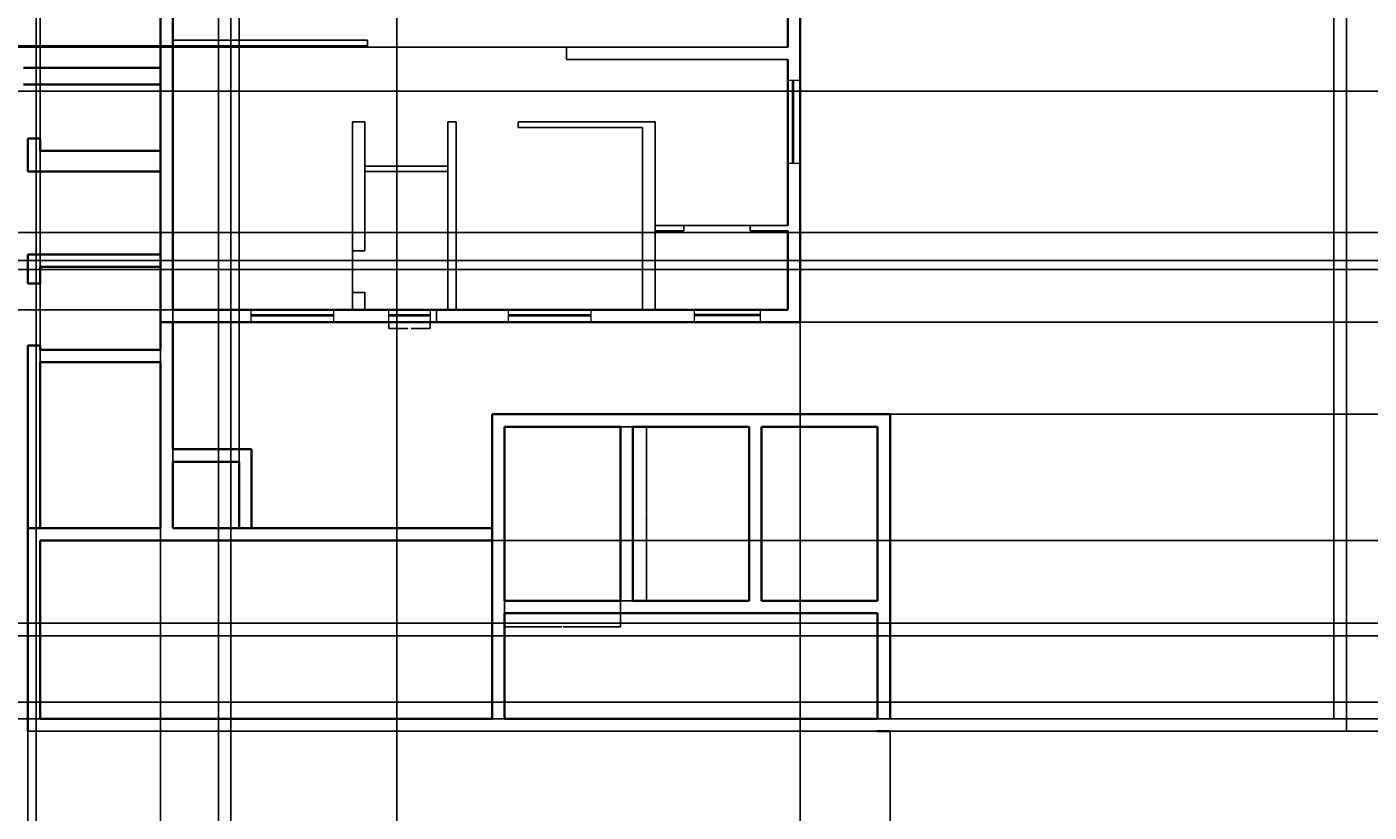
# Model space of a CAD drawing. Units: inches. Extents: x 2029 to 8798, y 1998 to 6373.
# Tile 5 of 11: x 2855 to 3826, y 4599 to 5168. Entities that reach past the tile are written whole.
import ezdxf

# ---------------------------------------------------------------- set-up
doc = ezdxf.new("R2010")
doc.units = ezdxf.units.IN
for name, color, linetype, lineweight in [('A-ANNO-DIMS', 2, 'Continuous', 18), ('A-GLAZ', 4, 'Continuous', 18), ('A-WALL-CIRC', 7, 'Continuous', 25), ('A-WALL-CORE', 7, 'Continuous', 35), ('A-WALL-EXTR', 7, 'Continuous', 35), ('A-WALL-INTR', 7, 'Continuous', 25)]:
    doc.layers.add(name, color=color, linetype=linetype, lineweight=lineweight)
doc.styles.get("Standard").update_dxf_attribs({"font": 'arial.ttf'})
doc.dimstyles.get("Standard").update_dxf_attribs({"dimtxt": 0.18, "dimasz": 0.18, "dimexe": 0.18, "dimexo": 0.0625, "dimgap": 0.09, "dimtad": 0, "dimtih": 1, "dimtoh": 1, "dimdec": 4, "dimzin": 0, "dimdsep": 46, "dimtxsty": 'Standard', "dimcen": 0.09, "dimadec": 0, "dimazin": 0, "dimtfac": 1, "dimtdec": 4, "dimtofl": 0, "dimtmove": 0, "dimatfit": 3, "dimfxl": 1, "dimtolj": 1, "dimtzin": 0, "dimarcsym": 0})

# ---------------------------------------------------------------- blocks, each defined once
blk = doc.blocks.new('WIN-60')
for p, q in [((0, 0), (0, 9)), ((0, 4.5), (60, 4.5)), ((0, 3.5), (60, 3.5)), ((60, 9), (60, 0))]:
    blk.add_line(p, q)
blk = doc.blocks.new('WIN-48')
for p, q in [((0, 48), (9, 48)), ((4.5, 48), (4.5, 0)), ((5.5, 48), (5.5, 0)), ((9, 0), (0, 0))]:
    blk.add_line(p, q)
blk = doc.blocks.new('WIN-30')
for p, q in [((0, 0), (0, 9)), ((0, 5.5), (30, 5.5)), ((0, 4.5), (30, 4.5)), ((30, 9), (30, 0))]:
    blk.add_line(p, q)
blk = doc.blocks.new('CORE-BAY-84X126')
for p, q in [((0, 126), (0, 0)), ((84, 126), (0, 126)), ((84, 126), (0, 126)), ((84, 0), (84, 126)), ((0, 0), (84, 0))]:
    blk.add_line(p, q)
blk = doc.blocks.new('*D21')
at = {"layer": 'A-ANNO-DIMS', "color": 0, "lineweight": -2, "transparency": 16777216}
for p, q in [((3116.78, 4953.93), (3116.78, 4949.31)), ((3146.78, 4953.93), (3146.78, 4949.31)), ((3116.96, 4949.49), (3130.66, 4949.49)), ((3146.6, 4949.49), (3132.9, 4949.49))]:
    blk.add_line(p, q, dxfattribs=at)
at = {"layer": 'A-ANNO-DIMS', "color": 0, "transparency": 16777216}
for points in [[(3116.96, 4949.52), (3116.96, 4949.46), (3116.78, 4949.49)], [(3146.6, 4949.52), (3146.6, 4949.46), (3146.78, 4949.49)]]:
    blk.add_solid(points, dxfattribs=at)
at = {"layer": 'Defpoints', "color": 0, "transparency": 16777216}
for p in [(3116.78, 4953.99), (3146.78, 4953.99), (3146.78, 4949.49)]:
    blk.add_point(p, dxfattribs=at)
at = {"layer": 'A-ANNO-DIMS', "color": 0, "transparency": 16777216, "insert": (3131.78, 4949.49), "char_height": 0.18, "attachment_point": 5}
blk.add_mtext('\\A1;WINDOW 30 TYP.', dxfattribs=at)
blk = doc.blocks.new('*D22')
at = {"layer": 'A-ANNO-DIMS', "color": 0, "lineweight": -2, "transparency": 16777216}
for p, q in [((3146.85, 4962.99), (3151.46, 4962.99)), ((3146.85, 4953.99), (3151.46, 4953.99)), ((3151.28, 4962.81), (3151.28, 4958.67)), ((3151.28, 4954.17), (3151.28, 4958.31))]:
    blk.add_line(p, q, dxfattribs=at)
at = {"layer": 'A-ANNO-DIMS', "color": 0, "transparency": 16777216}
for points in [[(3151.25, 4962.81), (3151.31, 4962.81), (3151.28, 4962.99)], [(3151.25, 4954.17), (3151.31, 4954.17), (3151.28, 4953.99)]]:
    blk.add_solid(points, dxfattribs=at)
at = {"layer": 'Defpoints', "color": 0, "transparency": 16777216}
for p in [(3146.78, 4962.99), (3146.78, 4953.99), (3151.28, 4962.99)]:
    blk.add_point(p, dxfattribs=at)
at = {"layer": 'A-ANNO-DIMS', "color": 0, "transparency": 16777216, "insert": (3151.28, 4958.49), "char_height": 0.18, "attachment_point": 5}
blk.add_mtext('\\A1;9 TYP.', dxfattribs=at)
blk = doc.blocks.new('*D27')
at = {"layer": 'A-ANNO-DIMS', "color": 0, "lineweight": -2, "transparency": 16777216}
for p, q in [((3284.59, 4878.3), (3303.61, 4878.3)), ((3303.43, 4878.12), (3303.43, 4815.48)), ((3303.43, 4752.48), (3303.43, 4815.12)), ((3284.59, 4752.3), (3303.61, 4752.3))]:
    blk.add_line(p, q, dxfattribs=at)
at = {"layer": 'A-ANNO-DIMS', "color": 0, "transparency": 16777216}
for points in [[(3303.4, 4878.12), (3303.46, 4878.12), (3303.43, 4878.3)], [(3303.4, 4752.48), (3303.46, 4752.48), (3303.43, 4752.3)]]:
    blk.add_solid(points, dxfattribs=at)
at = {"layer": 'Defpoints', "color": 0, "transparency": 16777216}
for p in [(3284.53, 4878.3), (3303.43, 4878.3), (3284.53, 4752.3)]:
    blk.add_point(p, dxfattribs=at)
at = {"layer": 'A-ANNO-DIMS', "color": 0, "transparency": 16777216, "insert": (3303.43, 4815.3), "char_height": 0.18, "attachment_point": 5}
blk.add_mtext('\\A1;CORE BAY 126 TYP.', dxfattribs=at)
blk = doc.blocks.new('*D28')
at = {"layer": 'A-ANNO-DIMS', "color": 0, "lineweight": -2, "transparency": 16777216}
for p, q in [((3200.53, 4752.24), (3200.53, 4733.22)), ((3284.53, 4752.24), (3284.53, 4733.22)), ((3200.71, 4733.4), (3242, 4733.4)), ((3284.35, 4733.4), (3243.06, 4733.4))]:
    blk.add_line(p, q, dxfattribs=at)
at = {"layer": 'A-ANNO-DIMS', "color": 0, "transparency": 16777216}
for points in [[(3200.71, 4733.43), (3200.71, 4733.37), (3200.53, 4733.4)], [(3284.35, 4733.43), (3284.35, 4733.37), (3284.53, 4733.4)]]:
    blk.add_solid(points, dxfattribs=at)
at = {"layer": 'Defpoints', "color": 0, "transparency": 16777216}
for p in [(3200.53, 4752.3), (3284.53, 4752.3), (3284.53, 4733.4)]:
    blk.add_point(p, dxfattribs=at)
at = {"layer": 'A-ANNO-DIMS', "color": 0, "transparency": 16777216, "insert": (3242.53, 4733.4), "char_height": 0.18, "attachment_point": 5}
blk.add_mtext('\\A1;84 TYP.', dxfattribs=at)
blk = doc.blocks.new('*D54')
at = {"layer": 'A-ANNO-DIMS', "color": 0, "lineweight": -2, "transparency": 16777216}
for p, q in [((2861.54, 4219.05), (2861.54, 6372.54)), ((2861.72, 6372.36), (2927.26, 6372.36)), ((2993.36, 6372.36), (2927.82, 6372.36)), ((2993.54, 4219.05), (2993.54, 6372.54))]:
    blk.add_line(p, q, dxfattribs=at)
at = {"layer": 'A-ANNO-DIMS', "color": 0, "transparency": 16777216}
for points in [[(2861.72, 6372.39), (2861.72, 6372.33), (2861.54, 6372.36)], [(2993.36, 6372.39), (2993.36, 6372.33), (2993.54, 6372.36)]]:
    blk.add_solid(points, dxfattribs=at)
at = {"layer": 'Defpoints', "color": 0, "transparency": 16777216}
for p in [(2993.54, 6372.36), (2861.54, 4218.99), (2993.54, 4218.99)]:
    blk.add_point(p, dxfattribs=at)
at = {"layer": 'A-ANNO-DIMS', "color": 0, "transparency": 16777216, "insert": (2927.54, 6372.36), "char_height": 0.18, "attachment_point": 5}
blk.add_mtext('\\A1;132', dxfattribs=at)
blk = doc.blocks.new('*D55')
at = {"layer": 'A-ANNO-DIMS', "color": 0, "lineweight": -2, "transparency": 16777216}
for p, q in [((3002.54, 4219.05), (3002.54, 6372.54)), ((3002.72, 6372.36), (3062.26, 6372.36)), ((3122.36, 6372.36), (3062.82, 6372.36)), ((3122.54, 4219.05), (3122.54, 6372.54))]:
    blk.add_line(p, q, dxfattribs=at)
at = {"layer": 'A-ANNO-DIMS', "color": 0, "transparency": 16777216}
for points in [[(3002.72, 6372.39), (3002.72, 6372.33), (3002.54, 6372.36)], [(3122.36, 6372.39), (3122.36, 6372.33), (3122.54, 6372.36)]]:
    blk.add_solid(points, dxfattribs=at)
at = {"layer": 'Defpoints', "color": 0, "transparency": 16777216}
for p in [(3122.54, 6372.36), (3002.54, 4218.99), (3122.54, 4218.99)]:
    blk.add_point(p, dxfattribs=at)
at = {"layer": 'A-ANNO-DIMS', "color": 0, "transparency": 16777216, "insert": (3062.54, 6372.36), "char_height": 0.18, "attachment_point": 5}
blk.add_mtext('\\A1;120', dxfattribs=at)
blk = doc.blocks.new('*D59')
at = {"layer": 'A-ANNO-DIMS', "color": 0, "lineweight": -2, "transparency": 16777216}
for p, q in [((2951.53, 4953.93), (2951.53, 4031.06)), ((3414.53, 4953.93), (3414.53, 4031.06)), ((2951.71, 4031.24), (3182.74, 4031.24)), ((3414.35, 4031.24), (3183.32, 4031.24))]:
    blk.add_line(p, q, dxfattribs=at)
at = {"layer": 'A-ANNO-DIMS', "color": 0, "transparency": 16777216}
for points in [[(2951.71, 4031.27), (2951.71, 4031.21), (2951.53, 4031.24)], [(3414.35, 4031.27), (3414.35, 4031.21), (3414.53, 4031.24)]]:
    blk.add_solid(points, dxfattribs=at)
at = {"layer": 'Defpoints', "color": 0, "transparency": 16777216}
for p in [(2951.53, 4953.99), (3414.53, 4953.99), (3414.53, 4031.24)]:
    blk.add_point(p, dxfattribs=at)
at = {"layer": 'A-ANNO-DIMS', "color": 0, "transparency": 16777216, "insert": (3183.03, 4031.24), "char_height": 0.18, "attachment_point": 5}
blk.add_mtext('\\A1;463', dxfattribs=at)
blk = doc.blocks.new('*D60')
at = {"layer": 'A-ANNO-DIMS', "color": 0, "lineweight": -2, "transparency": 16777216}
for p, q in [((3414.59, 5346.99), (4503.7, 5346.99)), ((4503.52, 5346.81), (4503.52, 5150.67)), ((4503.52, 4954.17), (4503.52, 5150.31)), ((3414.59, 4953.99), (4503.7, 4953.99))]:
    blk.add_line(p, q, dxfattribs=at)
at = {"layer": 'A-ANNO-DIMS', "color": 0, "transparency": 16777216}
for points in [[(4503.49, 5346.81), (4503.55, 5346.81), (4503.52, 5346.99)], [(4503.49, 4954.17), (4503.55, 4954.17), (4503.52, 4953.99)]]:
    blk.add_solid(points, dxfattribs=at)
at = {"layer": 'Defpoints', "color": 0, "transparency": 16777216}
for p in [(3414.53, 5346.99), (4503.52, 5346.99), (3414.53, 4953.99)]:
    blk.add_point(p, dxfattribs=at)
at = {"layer": 'A-ANNO-DIMS', "color": 0, "transparency": 16777216, "insert": (4503.52, 5150.49), "char_height": 0.18, "attachment_point": 5}
blk.add_mtext('\\A1;393', dxfattribs=at)
blk = doc.blocks.new('*D65')
at = {"layer": 'A-ANNO-DIMS', "color": 0, "lineweight": -2, "transparency": 16777216}
for p, q in [((3405.47, 5337.99), (2029.61, 5337.99)), ((2029.79, 5337.81), (2029.79, 5245.67)), ((2029.79, 5153.17), (2029.79, 5245.31)), ((3405.47, 5152.99), (2029.61, 5152.99))]:
    blk.add_line(p, q, dxfattribs=at)
at = {"layer": 'A-ANNO-DIMS', "color": 0, "transparency": 16777216}
for points in [[(2029.76, 5337.81), (2029.82, 5337.81), (2029.79, 5337.99)], [(2029.76, 5153.17), (2029.82, 5153.17), (2029.79, 5152.99)]]:
    blk.add_solid(points, dxfattribs=at)
at = {"layer": 'Defpoints', "color": 0, "transparency": 16777216}
for p in [(2029.79, 5337.99), (3405.53, 5337.99), (3405.53, 5152.99)]:
    blk.add_point(p, dxfattribs=at)
at = {"layer": 'A-ANNO-DIMS', "color": 0, "transparency": 16777216, "insert": (2029.79, 5245.49), "char_height": 0.18, "attachment_point": 5}
blk.add_mtext('\\A1;185', dxfattribs=at)
blk = doc.blocks.new('*D66')
at = {"layer": 'A-ANNO-DIMS', "color": 0, "lineweight": -2, "transparency": 16777216}
for p, q in [((2960.47, 5153.99), (2029.61, 5153.99)), ((2029.79, 5153.81), (2029.79, 5058.67)), ((2029.79, 4963.17), (2029.79, 5058.31)), ((2960.47, 4962.99), (2029.61, 4962.99))]:
    blk.add_line(p, q, dxfattribs=at)
at = {"layer": 'A-ANNO-DIMS', "color": 0, "transparency": 16777216}
for points in [[(2029.76, 5153.81), (2029.82, 5153.81), (2029.79, 5153.99)], [(2029.76, 4963.17), (2029.82, 4963.17), (2029.79, 4962.99)]]:
    blk.add_solid(points, dxfattribs=at)
at = {"layer": 'Defpoints', "color": 0, "transparency": 16777216}
for p in [(2029.79, 5153.99), (2960.53, 5153.99), (2960.53, 4962.99)]:
    blk.add_point(p, dxfattribs=at)
at = {"layer": 'A-ANNO-DIMS', "color": 0, "transparency": 16777216, "insert": (2029.79, 5058.49), "char_height": 0.18, "attachment_point": 5}
blk.add_mtext('\\A1;191', dxfattribs=at)
blk = doc.blocks.new('*D67')
at = {"layer": 'A-ANNO-DIMS', "color": 0, "lineweight": -2, "transparency": 16777216}
for p, q in [((2855.53, 4657.93), (2855.53, 4031.06)), ((3479.53, 4657.93), (3479.53, 4031.06)), ((2855.71, 4031.24), (3167.24, 4031.24)), ((3479.35, 4031.24), (3167.82, 4031.24))]:
    blk.add_line(p, q, dxfattribs=at)
at = {"layer": 'A-ANNO-DIMS', "color": 0, "transparency": 16777216}
for points in [[(2855.71, 4031.27), (2855.71, 4031.21), (2855.53, 4031.24)], [(3479.35, 4031.27), (3479.35, 4031.21), (3479.53, 4031.24)]]:
    blk.add_solid(points, dxfattribs=at)
at = {"layer": 'Defpoints', "color": 0, "transparency": 16777216}
for p in [(2855.53, 4657.99), (3479.53, 4657.99), (3479.53, 4031.24)]:
    blk.add_point(p, dxfattribs=at)
at = {"layer": 'A-ANNO-DIMS', "color": 0, "transparency": 16777216, "insert": (3167.53, 4031.24), "char_height": 0.18, "attachment_point": 5}
blk.add_mtext('\\A1;624', dxfattribs=at)
blk = doc.blocks.new('*D68')
at = {"layer": 'A-ANNO-DIMS', "color": 0, "lineweight": -2, "transparency": 16777216}
for p, q in [((3479.59, 4887.3), (4503.7, 4887.3)), ((4503.52, 4887.12), (4503.52, 4772.83)), ((4503.52, 4658.17), (4503.52, 4772.46)), ((3479.59, 4657.99), (4503.7, 4657.99))]:
    blk.add_line(p, q, dxfattribs=at)
at = {"layer": 'A-ANNO-DIMS', "color": 0, "transparency": 16777216}
for points in [[(4503.49, 4887.12), (4503.55, 4887.12), (4503.52, 4887.3)], [(4503.49, 4658.17), (4503.55, 4658.17), (4503.52, 4657.99)]]:
    blk.add_solid(points, dxfattribs=at)
at = {"layer": 'Defpoints', "color": 0, "transparency": 16777216}
for p in [(3479.53, 4887.3), (4503.52, 4887.3), (3479.53, 4657.99)]:
    blk.add_point(p, dxfattribs=at)
at = {"layer": 'A-ANNO-DIMS', "color": 0, "transparency": 16777216, "insert": (4503.52, 4772.64), "char_height": 0.18, "attachment_point": 5}
blk.add_mtext('\\A1;229.3', dxfattribs=at)
blk = doc.blocks.new('*D69')
at = {"layer": 'A-ANNO-DIMS', "color": 0, "lineweight": -2, "transparency": 16777216}
for p, q in [((3414.59, 4953.99), (4503.7, 4953.99)), ((4503.52, 4953.81), (4503.52, 4920.83)), ((4503.52, 4887.48), (4503.52, 4920.46)), ((3479.59, 4887.3), (4503.7, 4887.3))]:
    blk.add_line(p, q, dxfattribs=at)
at = {"layer": 'A-ANNO-DIMS', "color": 0, "transparency": 16777216}
for points in [[(4503.49, 4953.81), (4503.55, 4953.81), (4503.52, 4953.99)], [(4503.49, 4887.48), (4503.55, 4887.48), (4503.52, 4887.3)]]:
    blk.add_solid(points, dxfattribs=at)
at = {"layer": 'Defpoints', "color": 0, "transparency": 16777216}
for p in [(3414.53, 4953.99), (3479.53, 4887.3), (4503.52, 4887.3)]:
    blk.add_point(p, dxfattribs=at)
at = {"layer": 'A-ANNO-DIMS', "color": 0, "transparency": 16777216, "insert": (4503.52, 4920.64), "char_height": 0.18, "attachment_point": 5}
blk.add_mtext('\\A1;66.69', dxfattribs=at)
blk = doc.blocks.new('*D88')
at = {"layer": 'A-ANNO-DIMS', "color": 0, "lineweight": -2, "transparency": 16777216}
for p, q in [((2142.54, 4445.05), (2142.54, 6372.54)), ((2142.72, 6372.36), (3266.19, 6372.36)), ((4390.59, 6372.36), (3267.12, 6372.36)), ((4390.77, 4574.05), (4390.77, 6372.54))]:
    blk.add_line(p, q, dxfattribs=at)
at = {"layer": 'A-ANNO-DIMS', "color": 0, "transparency": 16777216}
for points in [[(2142.72, 6372.39), (2142.72, 6372.33), (2142.54, 6372.36)], [(4390.59, 6372.39), (4390.59, 6372.33), (4390.77, 6372.36)]]:
    blk.add_solid(points, dxfattribs=at)
at = {"layer": 'Defpoints', "color": 0, "transparency": 16777216}
for p in [(4390.77, 6372.36), (4390.77, 4573.99), (2142.54, 4444.99)]:
    blk.add_point(p, dxfattribs=at)
at = {"layer": 'A-ANNO-DIMS', "color": 0, "transparency": 16777216, "insert": (3266.65, 6372.36), "char_height": 0.18, "attachment_point": 5}
blk.add_mtext('\\A1;2248.2', dxfattribs=at)
blk = doc.blocks.new('*D91')
at = {"layer": 'A-ANNO-DIMS', "color": 0, "lineweight": -2, "transparency": 16777216}
for p, q in [((4095.32, 4736.09), (2029.61, 4736.09)), ((2029.79, 4735.91), (2029.79, 4707.78)), ((2029.79, 4679.27), (2029.79, 4707.41)), ((4095.32, 4679.09), (2029.61, 4679.09))]:
    blk.add_line(p, q, dxfattribs=at)
at = {"layer": 'A-ANNO-DIMS', "color": 0, "transparency": 16777216}
for points in [[(2029.76, 4735.91), (2029.82, 4735.91), (2029.79, 4736.09)], [(2029.76, 4679.27), (2029.82, 4679.27), (2029.79, 4679.09)]]:
    blk.add_solid(points, dxfattribs=at)
at = {"layer": 'Defpoints', "color": 0, "transparency": 16777216}
for p in [(2029.79, 4736.09), (4095.39, 4736.09), (4095.39, 4679.09)]:
    blk.add_point(p, dxfattribs=at)
at = {"layer": 'A-ANNO-DIMS', "color": 0, "transparency": 16777216, "insert": (2029.79, 4707.59), "char_height": 0.18, "attachment_point": 5}
blk.add_mtext('\\A1;57', dxfattribs=at)
blk = doc.blocks.new('*D106')
at = {"layer": 'A-ANNO-DIMS', "color": 0, "lineweight": -2, "transparency": 16777216}
for p, q in [((4325.32, 5121.09), (2029.61, 5121.09)), ((2029.79, 5120.91), (2029.79, 5056.78)), ((2029.79, 4992.27), (2029.79, 5056.41)), ((4325.32, 4992.09), (2029.61, 4992.09))]:
    blk.add_line(p, q, dxfattribs=at)
at = {"layer": 'A-ANNO-DIMS', "color": 0, "transparency": 16777216}
for points in [[(2029.76, 5120.91), (2029.82, 5120.91), (2029.79, 5121.09)], [(2029.76, 4992.27), (2029.82, 4992.27), (2029.79, 4992.09)]]:
    blk.add_solid(points, dxfattribs=at)
at = {"layer": 'Defpoints', "color": 0, "transparency": 16777216}
for p in [(4325.39, 5121.09), (2029.79, 4992.09), (4325.39, 4992.09)]:
    blk.add_point(p, dxfattribs=at)
at = {"layer": 'A-ANNO-DIMS', "color": 0, "transparency": 16777216, "insert": (2029.79, 5056.59), "char_height": 0.18, "attachment_point": 5}
blk.add_mtext('\\A1;129', dxfattribs=at)
blk = doc.blocks.new('*D110')
at = {"layer": 'A-ANNO-DIMS', "color": 0, "lineweight": -2, "transparency": 16777216}
for p, q in [((2723.6, 5018.96), (4503.7, 5018.96)), ((4503.52, 5018.78), (4503.52, 5008.93)), ((4503.52, 4998.71), (4503.52, 5008.56)), ((2723.6, 4998.53), (4503.7, 4998.53))]:
    blk.add_line(p, q, dxfattribs=at)
at = {"layer": 'A-ANNO-DIMS', "color": 0, "transparency": 16777216}
for points in [[(4503.49, 5018.78), (4503.55, 5018.78), (4503.52, 5018.96)], [(4503.49, 4998.71), (4503.55, 4998.71), (4503.52, 4998.53)]]:
    blk.add_solid(points, dxfattribs=at)
at = {"layer": 'Defpoints', "color": 0, "transparency": 16777216}
for p in [(2723.54, 5018.96), (2723.54, 4998.53), (4503.52, 4998.53)]:
    blk.add_point(p, dxfattribs=at)
at = {"layer": 'A-ANNO-DIMS', "color": 0, "transparency": 16777216, "insert": (4503.52, 5008.75), "char_height": 0.18, "attachment_point": 5}
blk.add_mtext('\\A1;20.425', dxfattribs=at)
blk = doc.blocks.new('*D111')
at = {"layer": 'A-ANNO-DIMS', "color": 0, "lineweight": -2, "transparency": 16777216}
for p, q in [((2723.6, 4726.96), (4503.7, 4726.96)), ((4503.52, 4726.78), (4503.52, 4697.16)), ((4503.52, 4667.17), (4503.52, 4696.79)), ((2723.6, 4666.99), (4503.7, 4666.99))]:
    blk.add_line(p, q, dxfattribs=at)
at = {"layer": 'A-ANNO-DIMS', "color": 0, "transparency": 16777216}
for points in [[(4503.49, 4726.78), (4503.55, 4726.78), (4503.52, 4726.96)], [(4503.49, 4667.17), (4503.55, 4667.17), (4503.52, 4666.99)]]:
    blk.add_solid(points, dxfattribs=at)
at = {"layer": 'Defpoints', "color": 0, "transparency": 16777216}
for p in [(2723.54, 4726.96), (4503.52, 4726.96), (2723.54, 4666.99)]:
    blk.add_point(p, dxfattribs=at)
at = {"layer": 'A-ANNO-DIMS', "color": 0, "transparency": 16777216, "insert": (4503.52, 4696.97), "char_height": 0.18, "attachment_point": 5}
blk.add_mtext('\\A1;59.97', dxfattribs=at)
blk = doc.blocks.new('*D113')
at = {"layer": 'A-ANNO-DIMS', "color": 0, "lineweight": -2, "transparency": 16777216}
for p, q in [((2864.59, 4795.99), (4503.7, 4795.99)), ((4503.52, 4795.81), (4503.52, 4731.67)), ((4503.52, 4667.17), (4503.52, 4731.31)), ((2864.59, 4666.99), (4503.7, 4666.99))]:
    blk.add_line(p, q, dxfattribs=at)
at = {"layer": 'A-ANNO-DIMS', "color": 0, "transparency": 16777216}
for points in [[(4503.49, 4795.81), (4503.55, 4795.81), (4503.52, 4795.99)], [(4503.49, 4667.17), (4503.55, 4667.17), (4503.52, 4666.99)]]:
    blk.add_solid(points, dxfattribs=at)
at = {"layer": 'Defpoints', "color": 0, "transparency": 16777216}
for p in [(2864.53, 4795.99), (4503.52, 4795.99), (2864.53, 4666.99)]:
    blk.add_point(p, dxfattribs=at)
at = {"layer": 'A-ANNO-DIMS', "color": 0, "transparency": 16777216, "insert": (4503.52, 4731.49), "char_height": 0.18, "attachment_point": 5}
blk.add_mtext('\\A1;129', dxfattribs=at)
blk = doc.blocks.new('*D114')
at = {"layer": 'A-ANNO-DIMS', "color": 0, "lineweight": -2, "transparency": 16777216}
for p, q in [((2864.53, 4805.05), (2864.53, 6372.54)), ((2864.71, 6372.36), (2907.81, 6372.36)), ((2951.35, 6372.36), (2908.25, 6372.36)), ((2951.53, 4805.05), (2951.53, 6372.54))]:
    blk.add_line(p, q, dxfattribs=at)
at = {"layer": 'A-ANNO-DIMS', "color": 0, "transparency": 16777216}
for points in [[(2864.71, 6372.39), (2864.71, 6372.33), (2864.53, 6372.36)], [(2951.35, 6372.39), (2951.35, 6372.33), (2951.53, 6372.36)]]:
    blk.add_solid(points, dxfattribs=at)
at = {"layer": 'Defpoints', "color": 0, "transparency": 16777216}
for p in [(2951.53, 6372.36), (2864.53, 4804.99), (2951.53, 4804.99)]:
    blk.add_point(p, dxfattribs=at)
at = {"layer": 'A-ANNO-DIMS', "color": 0, "transparency": 16777216, "insert": (2908.03, 6372.36), "char_height": 0.18, "attachment_point": 5}
blk.add_mtext('\\A1;87', dxfattribs=at)
blk = doc.blocks.new('*D115')
at = {"layer": 'A-ANNO-DIMS', "color": 0, "lineweight": -2, "transparency": 16777216}
for p, q in [((2960.53, 4805.05), (2960.53, 6372.54)), ((2960.71, 6372.36), (2984.31, 6372.36)), ((3008.35, 6372.36), (2984.75, 6372.36)), ((3008.53, 4805.05), (3008.53, 6372.54))]:
    blk.add_line(p, q, dxfattribs=at)
at = {"layer": 'A-ANNO-DIMS', "color": 0, "transparency": 16777216}
for points in [[(2960.71, 6372.39), (2960.71, 6372.33), (2960.53, 6372.36)], [(3008.35, 6372.39), (3008.35, 6372.33), (3008.53, 6372.36)]]:
    blk.add_solid(points, dxfattribs=at)
at = {"layer": 'Defpoints', "color": 0, "transparency": 16777216}
for p in [(3008.53, 6372.36), (2960.53, 4804.99), (3008.53, 4804.99)]:
    blk.add_point(p, dxfattribs=at)
at = {"layer": 'A-ANNO-DIMS', "color": 0, "transparency": 16777216, "insert": (2984.53, 6372.36), "char_height": 0.18, "attachment_point": 5}
blk.add_mtext('\\A1;48', dxfattribs=at)

msp = doc.modelspace()

# ---------------------------------------------------------------- linework, layer by layer
at = {"layer": 'A-GLAZ'}
for p, q in [((3414.5292, 5128.9636), (3414.5292, 5068.9636)), ((3076.9785, 4953.9886), (3016.9785, 4953.9886)), ((3146.7828, 4953.9886), (3116.7828, 4953.9886)), ((3263.2911, 4953.9886), (3203.2911, 4953.9886)), ((3385.7832, 4953.9886), (3337.7832, 4953.9886))]:
    msp.add_line(p, q, dxfattribs=at)
at = {"layer": 'A-WALL-CIRC'}
for p, q in [((3800.7657, 5069.4255), (3800.7657, 5497.3491)), ((3809.7657, 5497.3826), (3809.7657, 5069.4255)), ((3800.7657, 5069.4255), (3800.7657, 4666.9886)), ((3809.7657, 5069.4255), (3809.7657, 4657.9886)), ((3503.9638, 4666.9886), (3479.5292, 4666.9886)), ((3503.9638, 4666.9886), (3800.7657, 4666.9886)), ((3503.9638, 4657.9886), (2855.5292, 4657.9886)), ((3809.7657, 4657.9886), (3479.5292, 4657.9886)), ((3771.7657, 4657.9886), (3503.9638, 4657.9886)), ((3771.7657, 4657.9886), (3800.7657, 4657.9886)), ((3800.7657, 4657.9886), (3809.7657, 4657.9886))]:
    msp.add_line(p, q, dxfattribs=at)
at = {"layer": 'A-WALL-CORE'}
for p, q in [((2864.5292, 5137.9886), (2852.5292, 5137.9886)), ((2951.5292, 5137.9886), (2864.5292, 5137.9886)), ((2852.5292, 5125.9886), (2951.5292, 5125.9886)), ((2855.5292, 5074.9886), (2855.5292, 5086.9886)), ((2855.5292, 5086.9886), (2864.5292, 5086.9886)), ((2864.5292, 5086.9886), (2864.5292, 5077.9886)), ((2855.5292, 5062.9886), (2855.5292, 5074.9886)), ((2864.5292, 5077.9886), (2951.5292, 5077.9886)), ((2951.5292, 5062.9886), (2855.5292, 5062.9886)), ((2855.5292, 4993.9886), (2855.5292, 5002.9886)), ((2855.5292, 5002.9886), (2951.5292, 5002.9886)), ((2855.5292, 4981.9886), (2855.5292, 4993.9886)), ((2951.5292, 4993.9886), (2864.5292, 4993.9886)), ((2864.5292, 4993.9886), (2864.5292, 4981.9886)), ((2951.5292, 4933.9886), (2951.5292, 4993.9886)), ((2864.5292, 4981.9886), (2855.5292, 4981.9886)), ((2951.5292, 4933.9886), (2951.5292, 4957.9886)), ((2960.5292, 4933.9886), (2960.5292, 4953.9886)), ((2864.5292, 4936.9886), (2855.5292, 4936.9886)), ((2855.5292, 4936.9886), (2855.5292, 4924.9886)), ((2864.5292, 4933.9886), (2864.5292, 4936.9886)), ((2855.5292, 4804.9886), (2855.5292, 4924.9886)), ((2864.5292, 4933.9886), (2951.5292, 4933.9886)), ((2864.5292, 4924.9886), (2864.5292, 4804.9886)), ((2951.5292, 4924.9886), (2864.5292, 4924.9886)), ((2951.5292, 4804.9886), (2951.5292, 4924.9886)), ((2960.5292, 4933.9886), (2960.5292, 4861.9886)), ((3191.5292, 4752.2994), (3191.5292, 4887.2994)), ((3191.5292, 4887.2994), (3200.5292, 4887.2994)), ((3284.5292, 4887.2994), (3200.5292, 4887.2994)), ((3293.5292, 4887.2994), (3284.5292, 4887.2994)), ((3377.5292, 4887.2994), (3293.5292, 4887.2994)), ((3386.5292, 4887.2994), (3377.5292, 4887.2994)), ((3470.5292, 4887.2994), (3386.5292, 4887.2994)), ((3479.5292, 4887.2994), (3470.5292, 4887.2994)), ((3479.5292, 4887.2994), (3470.5292, 4887.2994)), ((3479.5292, 4803.2994), (3479.5292, 4887.2994)), ((3017.5292, 4861.9886), (2960.5292, 4861.9886)), ((3017.5292, 4852.9886), (3017.5292, 4861.9886)), ((2960.5292, 4804.9886), (2960.5292, 4852.9886)), ((2960.5292, 4852.9886), (3008.5292, 4852.9886)), ((2960.5292, 4852.9886), (2960.5292, 4804.9886)), ((3008.5292, 4852.9886), (3008.5292, 4804.9886)), ((3017.5292, 4804.9886), (3017.5292, 4852.9886)), ((2855.5292, 4795.9886), (2855.5292, 4804.9886)), ((2855.5292, 4804.9886), (2951.5292, 4804.9886)), ((2864.5292, 4804.9886), (2951.5292, 4804.9886)), ((2960.5292, 4804.9886), (3191.5292, 4804.9886)), ((3008.5292, 4804.9886), (3017.5292, 4804.9886)), ((3479.5292, 4743.2994), (3479.5292, 4803.2994)), ((2855.5292, 4666.9886), (2855.5292, 4795.9886)), ((2951.5292, 4795.9886), (2864.5292, 4795.9886)), ((2864.5292, 4795.9886), (2864.5292, 4666.9886)), ((3071.5292, 4795.9886), (2951.5292, 4795.9886)), ((3191.5292, 4795.9886), (3071.5292, 4795.9886)), ((3191.5292, 4666.9886), (3191.5292, 4795.9886)), ((3191.5292, 4666.9886), (3191.5292, 4753.9886)), ((3191.5292, 4752.2994), (3191.5292, 4666.9886)), ((3479.5292, 4752.2994), (3479.5292, 4666.9886)), ((3200.5292, 4666.9886), (3200.5292, 4743.2994)), ((3200.5292, 4743.2994), (3470.5292, 4743.2994)), ((3470.5292, 4666.9886), (3470.5292, 4743.2994)), ((2855.5292, 4666.9886), (2855.5292, 4657.9886)), ((3191.5292, 4666.9886), (2864.5292, 4666.9886)), ((3470.5292, 4666.9886), (3200.5292, 4666.9886)), ((3293.5292, 4666.9886), (3284.5292, 4666.9886)), ((3386.5292, 4666.9886), (3377.5292, 4666.9886)), ((3479.5292, 4657.9886), (3470.5292, 4657.9886))]:
    msp.add_line(p, q, dxfattribs=at)
at = {"layer": 'A-WALL-EXTR'}
for p, q in [((2951.5292, 5337.9886), (2951.5292, 4962.9886)), ((3414.5292, 4953.9886), (3414.5292, 5337.9886)), ((2960.5292, 5157.9886), (2960.5292, 5265.9886)), ((3405.5292, 5212.9886), (3405.5292, 5152.9886)), ((2960.5292, 5157.9886), (2960.5292, 5153.9886)), ((2960.5292, 4966.9886), (2960.5292, 5153.9886)), ((3405.5292, 5143.9886), (3405.5292, 5023.9886)), ((3405.5292, 5143.9886), (3405.5292, 5128.9636)), ((2951.5292, 5077.9886), (2951.5292, 5137.9886)), ((2951.5292, 5002.9886), (2951.5292, 5062.9886)), ((3405.5292, 5019.9886), (3405.5292, 4962.9886)), ((2951.5292, 4957.9886), (2951.5292, 4966.9886)), ((2960.5292, 4962.9886), (2960.5292, 4966.9886)), ((2951.5292, 4962.9886), (2951.5292, 4953.9886)), ((2951.5292, 4953.9886), (3405.5292, 4953.9886)), ((3405.5292, 4962.9886), (2960.5292, 4962.9886)), ((3090.5292, 4962.9886), (3076.9785, 4962.9886)), ((3099.5292, 4962.9886), (3090.5292, 4962.9886)), ((3159.5292, 4962.9886), (3146.7828, 4962.9886)), ((3300.5292, 4962.9886), (3165.5292, 4962.9886)), ((3300.5292, 4962.9886), (3263.2911, 4962.9886)), ((3405.5292, 4962.9886), (3309.5292, 4962.9886)), ((3405.5292, 4962.9886), (3385.7832, 4962.9886)), ((3405.5292, 4953.9886), (3414.5292, 4953.9886))]:
    msp.add_line(p, q, dxfattribs=at)
at = {"layer": 'A-WALL-INTR'}
for p, q in [((3096.5292, 5157.9886), (2960.5292, 5157.9886)), ((3092.5292, 5157.9886), (3092.5292, 5157.9886)), ((3092.5292, 5157.9886), (3101.5292, 5157.9886)), ((3096.5292, 5157.9886), (3101.5292, 5157.9886)), ((3101.5292, 5157.9886), (3101.5292, 5153.9886)), ((2960.5292, 5153.9886), (3096.5292, 5153.9886)), ((3101.5292, 5153.9886), (3096.5292, 5153.9886)), ((3254.5292, 5152.9886), (3245.5292, 5152.9886)), ((3245.5292, 5152.9886), (3245.5292, 5143.9886)), ((3405.5292, 5152.9886), (3254.5292, 5152.9886)), ((3245.5292, 5143.9886), (3405.5292, 5143.9886)), ((3090.5292, 5062.9886), (3090.5292, 5098.9886)), ((3090.5292, 5098.9886), (3099.5292, 5098.9886)), ((3099.5292, 5098.9886), (3099.5292, 5062.9886)), ((3165.5292, 5098.9886), (3159.5292, 5098.9886)), ((3159.5292, 5098.9886), (3159.5292, 4962.9886)), ((3159.5292, 5098.9886), (3159.5292, 5062.9886)), ((3165.5292, 4962.9886), (3165.5292, 5098.9886)), ((3309.5292, 5098.9886), (3210.5292, 5098.9886)), ((3210.5292, 5098.9886), (3210.5292, 5094.9886)), ((3210.5292, 5094.9886), (3300.5292, 5094.9886)), ((3300.5292, 5094.9886), (3300.5292, 4962.9886)), ((3309.5292, 4962.9886), (3309.5292, 5098.9886)), ((3090.5292, 4962.9886), (3090.5292, 5062.9886)), ((3099.5292, 5062.9886), (3099.5292, 5066.9886)), ((3099.5292, 5066.9886), (3159.5292, 5066.9886)), ((3159.5292, 5062.9886), (3099.5292, 5062.9886)), ((3099.5292, 5062.9886), (3099.5292, 5005.7062)), ((3405.5292, 5023.9886), (3309.5292, 5023.9886)), ((3309.5292, 5023.9886), (3309.5292, 5019.9886)), ((3309.5292, 5023.9886), (3330.3309, 5023.9886)), ((3330.3309, 5023.9886), (3330.3309, 5019.9886)), ((3378.3309, 5019.9886), (3378.3309, 5023.9886)), ((3309.5292, 5019.9886), (3330.3309, 5019.9886)), ((3378.3309, 5019.9886), (3405.5292, 5019.9886)), ((3099.5292, 5005.7062), (3090.5292, 5005.7062)), ((3090.5292, 5005.7062), (3090.5292, 4975.3922)), ((3090.5292, 4975.3922), (3099.5292, 4975.3922)), ((3099.5292, 4962.9886), (3099.5292, 4975.7062)), ((3099.5292, 4975.3922), (3099.5292, 4962.9886))]:
    msp.add_line(p, q, dxfattribs=at)

# ---------------------------------------------------------------- block references
at = {"layer": 'A-GLAZ', "extrusion": (0, 0, -1), "zscale": -1}
for name, p, rotation in [('WIN-60', (-3405.5292, 5068.9636), 90), ('WIN-60', (-3016.9785, 4962.9886), 180), ('WIN-60', (-3203.2911, 4962.9886), 180), ('WIN-48', (-3337.7832, 4953.9886), 90)]:
    msp.add_blockref(name, p, dxfattribs=dict(at, rotation=rotation))
at = {"layer": 'A-GLAZ'}
msp.add_blockref('WIN-30', (3116.7828, 4953.9886), dxfattribs=at)
at = {"layer": 'A-WALL-CORE'}
for p in [(3200.5292, 4752.2994), (3293.5292, 4752.2994), (3386.5292, 4752.2994)]:
    msp.add_blockref('CORE-BAY-84X126', p, dxfattribs=at)

# ---------------------------------------------------------------- dimensions: what is measured, and where the dimension line sits
at = {"layer": 'A-ANNO-DIMS'}
for base, p1, p2, override, picture, middle in [((4390.7657, 6372.3623), (2142.5398, 4444.9886), (4390.7657, 4573.9886), {"dimdec": 1, "dimlfac": 1, "dimrnd": 0, "dimzin": 0, "dimdsep": 46, "dimlunit": 2}, '*D88', (3266.6528, 6372.3623)), ((2993.5398, 6372.3623), (2861.5398, 4218.9886), (2993.5398, 4218.9886), {"dimdec": 0, "dimlfac": 1, "dimrnd": 0, "dimzin": 0, "dimdsep": 46, "dimlunit": 2}, '*D54', (2927.5398, 6372.3623)), ((2951.5292, 6372.3623), (2864.5292, 4804.9886), (2951.5292, 4804.9886), {"dimdec": 0, "dimlfac": 1, "dimrnd": 0, "dimzin": 0, "dimdsep": 46, "dimlunit": 2}, '*D114', (2908.0292, 6372.3623)), ((3008.5292, 6372.3623), (2960.5292, 4804.9886), (3008.5292, 4804.9886), {"dimdec": 0, "dimlfac": 1, "dimrnd": 0, "dimzin": 0, "dimdsep": 46, "dimlunit": 2}, '*D115', (2984.5292, 6372.3623)), ((3122.5398, 6372.3623), (3002.5398, 4218.9886), (3122.5398, 4218.9886), {"dimdec": 0, "dimlfac": 1, "dimrnd": 0, "dimzin": 0, "dimdsep": 46, "dimlunit": 2}, '*D55', (3062.5398, 6372.3623)), ((3414.5292, 4031.2386), (2951.5292, 4953.9886), (3414.5292, 4953.9886), {"dimdec": 0, "dimlfac": 1, "dimrnd": 0, "dimzin": 0, "dimdsep": 46, "dimlunit": 2}, '*D59', (3183.0292, 4031.2386)), ((3479.5292, 4031.2386), (2855.5292, 4657.9886), (3479.5292, 4657.9886), {"dimdec": 0, "dimlfac": 1, "dimrnd": 0, "dimzin": 0, "dimdsep": 46, "dimlunit": 2}, '*D67', (3167.5292, 4031.2386))]:
    dim = msp.add_linear_dim(base=base, p1=p1, p2=p2, dimstyle='Standard', override=override, dxfattribs=at)
    dim.commit()
    dim.dimension.update_dxf_attribs({"geometry": picture, "text_midpoint": middle})
for base, p1, p2, override, picture, middle in [((4503.5157, 5346.9886), (3414.5292, 4953.9886), (3414.5292, 5346.9886), {"dimdec": 0, "dimlfac": 1, "dimrnd": 0, "dimzin": 0, "dimdsep": 46, "dimlunit": 2}, '*D60', (4503.5157, 5150.4886)), ((2029.7898, 5337.9886), (3405.5292, 5152.9886), (3405.5292, 5337.9886), {"dimdec": 0, "dimlfac": 1, "dimrnd": 0, "dimzin": 0, "dimdsep": 46, "dimlunit": 2}, '*D65', (2029.7898, 5245.4886)), ((2029.7898, 5153.9886), (2960.5292, 4962.9886), (2960.5292, 5153.9886), {"dimdec": 0, "dimlfac": 1, "dimrnd": 0, "dimzin": 0, "dimdsep": 46, "dimlunit": 2}, '*D66', (2029.7898, 5058.4886)), ((2029.7898, 4992.0948), (4325.3869, 5121.0948), (4325.3869, 4992.0948), {"dimdec": 0, "dimlfac": 1, "dimrnd": 0, "dimzin": 0, "dimdsep": 46, "dimlunit": 2}, '*D106', (2029.7898, 5056.5948)), ((4503.5157, 4998.5338), (2723.5398, 5018.9585), (2723.5398, 4998.5338), {"dimdec": 3, "dimlfac": 1, "dimrnd": 0, "dimzin": 0, "dimdsep": 46, "dimlunit": 2}, '*D110', (4503.5157, 5008.7461)), ((4503.5157, 4887.2994), (3414.5292, 4953.9886), (3479.5292, 4887.2994), {"dimdec": 2, "dimlfac": 1, "dimrnd": 0, "dimzin": 0, "dimdsep": 46, "dimlunit": 2}, '*D69', (4503.5157, 4920.644)), ((4503.5157, 4887.2994), (3479.5292, 4657.9886), (3479.5292, 4887.2994), {"dimdec": 1, "dimlfac": 1, "dimrnd": 0, "dimzin": 0, "dimdsep": 46, "dimlunit": 2}, '*D68', (4503.5157, 4772.644)), ((4503.5157, 4795.9886), (2864.5292, 4666.9886), (2864.5292, 4795.9886), {"dimdec": 0, "dimlfac": 1, "dimrnd": 0, "dimzin": 0, "dimdsep": 46, "dimlunit": 2}, '*D113', (4503.5157, 4731.4886)), ((2029.7898, 4736.0948), (4095.3869, 4679.0948), (4095.3869, 4736.0948), {"dimdec": 0, "dimlfac": 1, "dimrnd": 0, "dimzin": 0, "dimdsep": 46, "dimlunit": 2}, '*D91', (2029.7898, 4707.5948)), ((4503.5157, 4726.9585), (2723.5398, 4666.9886), (2723.5398, 4726.9585), {"dimdec": 2, "dimlfac": 1, "dimrnd": 0, "dimzin": 0, "dimdsep": 46, "dimlunit": 2}, '*D111', (4503.5157, 4696.9735))]:
    dim = msp.add_linear_dim(base=base, p1=p1, p2=p2, angle=90, dimstyle='Standard', override=override, dxfattribs=at)
    dim.commit()
    dim.dimension.update_dxf_attribs({"geometry": picture, "text_midpoint": middle})
for base, p1, p2, text, picture, middle in [((3146.7828, 4949.4886), (3116.7828, 4953.9886), (3146.7828, 4953.9886), 'WINDOW <> TYP.', '*D21', (3131.7828, 4949.4886)), ((3284.5292, 4733.3994), (3200.5292, 4752.2994), (3284.5292, 4752.2994), '<> TYP.', '*D28', (3242.5292, 4733.3994))]:
    dim = msp.add_linear_dim(base=base, p1=p1, p2=p2, text=text, dimstyle='Standard', override={"dimdec": 0, "dimlfac": 1, "dimrnd": 0, "dimzin": 0, "dimdsep": 46, "dimlunit": 2}, dxfattribs=at)
    dim.commit()
    dim.dimension.update_dxf_attribs({"geometry": picture, "text_midpoint": middle})
for base, p1, p2, text, picture, middle in [((3151.2828, 4962.9886), (3146.7828, 4953.9886), (3146.7828, 4962.9886), '<> TYP.', '*D22', (3151.2828, 4958.4886)), ((3303.4292, 4878.2994), (3284.5292, 4752.2994), (3284.5292, 4878.2994), 'CORE BAY <> TYP.', '*D27', (3303.4292, 4815.2994))]:
    dim = msp.add_linear_dim(base=base, p1=p1, p2=p2, angle=90, text=text, dimstyle='Standard', override={"dimdec": 0, "dimlfac": 1, "dimrnd": 0, "dimzin": 0, "dimdsep": 46, "dimlunit": 2}, dxfattribs=at)
    dim.commit()
    dim.dimension.update_dxf_attribs({"geometry": picture, "text_midpoint": middle})

doc.saveas('drawing.dxf')
